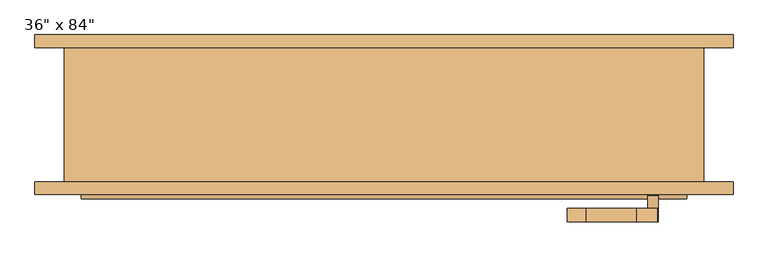
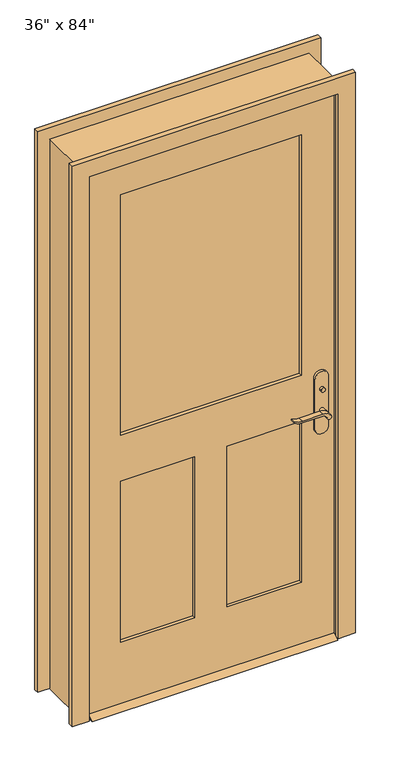
"""IFC4 building model written with IfcOpenShell, lengths in millimetres: door geometry."""

from ifc_helpers import new_model, si_unit, point, frame, frame_2d, origin, place, context, project, spatial, polyline, circle_curve, trimmed, segment, composite_curve, outline, extrude, faceted_brep, source, transform, mapped, element, save


def door_e879f077(model_context):
    return source(origin(), model_context, "Body", "SolidModel", [
        extrude(outline(polyline([(-63.5, 12.7), (-38.1, 0.0), (-123.825, 0.0), (-98.425, 12.7), (-63.5, 12.7)])), frame((-457.2, 0.0, 0.0), z_axis=(1.0, 0.0, 0.0), x_axis=(0.0, 1.0, 0.0)), (0.0, 0.0, 1.0), 914.4),
        extrude(outline(polyline([(411.4, -43.5), (411.4, -53.5), (401.4, -53.5), (401.4, -43.5), (411.4, -43.5)])), frame((0.0, 0.0, 981.9), z_axis=(0.0, 0.0, 1.0), x_axis=(1.0, 0.0, 0.0)), (0.0, 0.0, 1.0), 30.0),
        extrude(outline(composite_curve([segment(trimmed(circle_curve(frame_2d((996.9, 406.4)), 8.0), [point((996.9, 398.4))], [point((996.9, 414.4))], False, "CARTESIAN"), True, "CONTINUOUS"), segment(trimmed(circle_curve(frame_2d((996.9, 406.4)), 8.0), [point((996.9, 414.4))], [point((996.9, 398.4))], False, "CARTESIAN"), True, "CONTINUOUS")], self_intersect=False)), frame((0.0, -118.425, 0.0), z_axis=(0.0, 1.0, 0.0), x_axis=(0.0, 0.0, 1.0)), (0.0, 0.0, 1.0), 10.0),
        extrude(outline(composite_curve([segment(trimmed(circle_curve(frame_2d((897.1555521, 382.7324871)), 37.2832219), [point((919.0523287, 412.9081363))], [point((934.4, 381.0325667))], False, "CARTESIAN"), True, "CONTINUOUS"), segment(polyline([(934.4, 381.0325667), (934.4, 304.7564091)]), True, "CONTINUOUS"), segment(trimmed(circle_curve(frame_2d((1017.6850638, 304.8227909)), 83.2850902), [point((934.4, 304.7564091))], [point((939.4, 276.4))], True, "CARTESIAN"), True, "CONTINUOUS"), segment(polyline([(939.4, 276.4), (936.6135558, 276.4)]), True, "CONTINUOUS"), segment(trimmed(circle_curve(frame_2d((986.6709207, 308.3396612)), 59.3791355), [point((936.6135558, 276.4))], [point((927.4, 304.7564091))], False, "CARTESIAN"), True, "CONTINUOUS"), segment(polyline([(927.4, 304.7564091), (927.4, 381.0138099)]), True, "CONTINUOUS"), segment(trimmed(circle_curve(frame_2d((909.2738613, 381.0138099)), 18.1261387), [point((927.4, 381.0138099))], [point((914.4, 398.4))], True, "CARTESIAN"), True, "CONTINUOUS"), segment(trimmed(circle_curve(frame_2d((914.4, 406.4)), 8.0), [point((914.4, 398.4))], [point((919.0523287, 412.9081363))], False, "CARTESIAN"), True, "CONTINUOUS")], self_intersect=False)), frame((0.0, -23.5, 0.0), z_axis=(0.0, 1.0, 0.0), x_axis=(0.0, 0.0, 1.0)), (0.0, 0.0, 1.0), 20.0),
        extrude(outline(composite_curve([segment(trimmed(circle_curve(frame_2d((914.4, 406.4)), 8.0), [point((914.3999903, 398.4))], [point((919.0523287, 412.9081363))], False, "CARTESIAN"), True, "CONTINUOUS"), segment(trimmed(circle_curve(frame_2d((897.1555521, 382.7324871)), 37.2832219), [point((919.0523287, 412.9081363))], [point((934.4, 381.0325667))], False, "CARTESIAN"), True, "CONTINUOUS"), segment(polyline([(934.4, 381.0325667), (934.4, 304.7564091)]), True, "CONTINUOUS"), segment(trimmed(circle_curve(frame_2d((1017.6850638, 304.8227909)), 83.2850902), [point((934.4, 304.7564091))], [point((939.4, 276.4))], True, "CARTESIAN"), True, "CONTINUOUS"), segment(polyline([(939.4, 276.4), (936.6135558, 276.4)]), True, "CONTINUOUS"), segment(trimmed(circle_curve(frame_2d((986.6709207, 308.3396612)), 59.3791355), [point((936.6135558, 276.4))], [point((927.4, 304.7564091))], False, "CARTESIAN"), True, "CONTINUOUS"), segment(polyline([(927.4, 304.7564091), (927.4, 381.0138122)]), True, "CONTINUOUS"), segment(trimmed(circle_curve(frame_2d((909.2738682, 381.0138122)), 18.1261318), [point((927.4, 381.0138122))], [point((914.3999903, 398.4))], True, "CARTESIAN"), True, "CONTINUOUS")], self_intersect=False)), frame((0.0, -158.425, 0.0), z_axis=(0.0, 1.0, 0.0), x_axis=(0.0, 0.0, 1.0)), (0.0, 0.0, 1.0), 20.0),
        extrude(outline(composite_curve([segment(trimmed(circle_curve(frame_2d((914.4, 406.4)), 8.0), [point((914.4, 398.4))], [point((914.4, 414.4))], False, "CARTESIAN"), True, "CONTINUOUS"), segment(trimmed(circle_curve(frame_2d((914.4, 406.4)), 8.0), [point((914.4, 414.4))], [point((914.4, 398.4))], False, "CARTESIAN"), True, "CONTINUOUS")], self_intersect=False)), frame((0.0, -53.5, 0.0), z_axis=(0.0, 1.0, 0.0), x_axis=(0.0, 0.0, 1.0)), (0.0, 0.0, 1.0), 30.0),
        extrude(outline(composite_curve([segment(trimmed(circle_curve(frame_2d((914.4, 406.4)), 8.0), [point((914.4, 398.4))], [point((914.4, 414.4))], False, "CARTESIAN"), True, "CONTINUOUS"), segment(trimmed(circle_curve(frame_2d((914.4, 406.4)), 8.0), [point((914.4, 414.4))], [point((914.4, 398.4))], False, "CARTESIAN"), True, "CONTINUOUS")], self_intersect=False)), frame((0.0, -138.425, 0.0), z_axis=(0.0, 1.0, 0.0), x_axis=(0.0, 0.0, 1.0)), (0.0, 0.0, 1.0), 30.0),
        extrude(outline(composite_curve([segment(polyline([(844.4, 431.4), (1039.4, 431.4)]), True, "CONTINUOUS"), segment(trimmed(circle_curve(frame_2d((1039.4, 406.4)), 25.0), [point((1039.4, 431.4))], [point((1039.4, 381.4))], False, "CARTESIAN"), True, "CONTINUOUS"), segment(polyline([(1039.4, 381.4), (844.4, 381.4)]), True, "CONTINUOUS"), segment(trimmed(circle_curve(frame_2d((844.4, 406.4)), 25.0), [point((844.4, 381.4))], [point((844.4, 431.4))], False, "CARTESIAN"), True, "CONTINUOUS")], self_intersect=False)), frame((0.0, -63.5, 0.0), z_axis=(0.0, 1.0, 0.0), x_axis=(0.0, 0.0, 1.0)), (0.0, 0.0, 1.0), 10.0),
        extrude(outline(composite_curve([segment(polyline([(844.4, 431.4), (1039.4, 431.4)]), True, "CONTINUOUS"), segment(trimmed(circle_curve(frame_2d((1039.4, 406.4)), 25.0), [point((1039.4, 431.4))], [point((1039.4, 381.4))], False, "CARTESIAN"), True, "CONTINUOUS"), segment(polyline([(1039.4, 381.4), (844.4, 381.4)]), True, "CONTINUOUS"), segment(trimmed(circle_curve(frame_2d((844.4, 406.4)), 25.0), [point((844.4, 381.4))], [point((844.4, 431.4))], False, "CARTESIAN"), True, "CONTINUOUS")], self_intersect=False)), frame((0.0, -108.425, 0.0), z_axis=(0.0, 1.0, 0.0), x_axis=(0.0, 0.0, 1.0)), (0.0, 0.0, 1.0), 10.0),
        extrude(outline(polyline([(2133.6, -457.2), (12.7, -457.2), (12.7, 457.2), (2133.6, 457.2), (2133.6, -457.2)]), holes=[polyline([(1066.8, -336.55), (2012.95, -336.55), (2012.95, 336.55), (1066.8, 336.55), (1066.8, -336.55)]), polyline([(885.825, -60.325), (254.0, -60.325), (254.0, -336.55), (885.825, -336.55), (885.825, -60.325)]), polyline([(885.825, 336.55), (254.0, 336.55), (254.0, 60.325), (885.825, 60.325), (885.825, 336.55)])]), frame((0.0, -98.425, 0.0), z_axis=(0.0, 1.0, 0.0), x_axis=(0.0, 0.0, 1.0)), (0.0, 0.0, 1.0), 34.925),
        faceted_brep([(482.6, -98.425, 0.0), (457.2, -98.425, 0.0), (457.2, -63.5, 0.0), (444.5, -63.5, 0.0), (444.5, -28.575, 0.0), (457.2, -28.575, 0.0), (457.2, 104.775, 0.0), (482.6, 104.775, 0.0), (482.6, 104.775, 2159.0), (482.6, -98.425, 2159.0), (457.2, 104.775, 2133.6), (-457.2, 104.775, 2133.6), (-457.2, 104.775, 0.0), (-482.6, 104.775, 0.0), (-482.6, 104.775, 2159.0), (457.2, -28.575, 2133.6), (444.5, -28.575, 2120.9), (-444.5, -28.575, 2120.9), (-444.5, -28.575, 0.0), (-457.2, -28.575, 0.0), (-457.2, -28.575, 2133.6), (444.5, -63.5, 2120.9), (457.2, -63.5, 2133.6), (-457.2, -63.5, 2133.6), (-457.2, -63.5, 0.0), (-444.5, -63.5, 0.0), (-444.5, -63.5, 2120.9), (457.2, -98.425, 2133.6), (-482.6, -98.425, 2159.0), (-482.6, -98.425, 0.0), (-457.2, -98.425, 0.0), (-457.2, -98.425, 2133.6)], [[[0, 1, 2, 3, 4, 5, 6, 7]], [[7, 8, 9, 0]], [[6, 10, 11, 12, 13, 14, 8, 7]], [[5, 15, 10, 6]], [[4, 16, 17, 18, 19, 20, 15, 5]], [[3, 21, 16, 4]], [[2, 22, 23, 24, 25, 26, 21, 3]], [[1, 27, 22, 2]], [[0, 9, 28, 29, 30, 31, 27, 1]], [[8, 14, 28, 9]], [[15, 20, 11, 10]], [[21, 26, 17, 16]], [[27, 31, 23, 22]], [[29, 13, 12, 19, 18, 25, 24, 30]], [[14, 13, 29, 28]], [[20, 19, 12, 11]], [[26, 25, 18, 17]], [[31, 30, 24, 23]]]),
        extrude(outline(polyline([(-60.325, -75.1416667), (-60.325, -86.7833333), (-336.55, -86.7833333), (-336.55, -75.1416667), (-60.325, -75.1416667)])), frame((0.0, 0.0, 254.0), z_axis=(0.0, 0.0, 1.0), x_axis=(1.0, 0.0, 0.0)), (0.0, 0.0, 1.0), 631.825),
        extrude(outline(polyline([(336.55, -75.1416667), (336.55, -86.7833333), (60.325, -86.7833333), (60.325, -75.1416667), (336.55, -75.1416667)])), frame((0.0, 0.0, 254.0), z_axis=(0.0, 0.0, 1.0), x_axis=(1.0, 0.0, 0.0)), (0.0, 0.0, 1.0), 631.825),
        extrude(outline(polyline([(336.55, -77.47), (336.55, -84.455), (-336.55, -84.455), (-336.55, -77.47), (336.55, -77.47)])), frame((0.0, 0.0, 1066.8), z_axis=(0.0, 0.0, 1.0), x_axis=(1.0, 0.0, 0.0)), (0.0, 0.0, 1.0), 946.15),
        extrude(outline(polyline([(0.0, -463.55), (2139.95, -463.55), (2139.95, 463.55), (0.0, 463.55), (0.0, 527.05), (2203.45, 527.05), (2203.45, -527.05), (0.0, -527.05), (0.0, -463.55)])), frame((0.0, 104.775, 0.0), z_axis=(0.0, 1.0, 0.0), x_axis=(0.0, 0.0, 1.0)), (0.0, 0.0, 1.0), 19.05),
        extrude(outline(polyline([(0.0, -463.55), (2139.95, -463.55), (2139.95, 463.55), (0.0, 463.55), (0.0, 527.05), (2203.45, 527.05), (2203.45, -527.05), (0.0, -527.05), (0.0, -463.55)])), frame((0.0, -117.475, 0.0), z_axis=(0.0, 1.0, 0.0), x_axis=(0.0, 0.0, 1.0)), (0.0, 0.0, 1.0), 19.05),
    ])


if __name__ == "__main__":
    model = new_model("IFC4")
    model_context = context("Model", 3, world=origin())
    ifc_project = project(units=[si_unit("LENGTHUNIT", "METRE", prefix="MILLI")], contexts=[model_context])
    site = spatial("IfcSite", under=ifc_project)
    building = spatial("IfcBuilding", under=site)
    placement = place(None, origin())
    door_shape = door_e879f077(model_context)
    element("IfcDoor", 1, ObjectType="36\" x 84\"", at=placement, inside=building, context=model_context, shape_type="MappedRepresentation", body=[
        mapped(door_shape, transform((0.0, 0.0, 0.0), x_axis=(1.0, 0.0, 0.0), y_axis=(0.0, 1.0, 0.0), z_axis=(0.0, 0.0, 1.0))),
    ])
    save(model, "model.ifc")

# Revit data of these elements
# Type "36\" x 84\""
#   Type Mark = "15"
#   Assembly Code = "B2030100"
#   Analytic Construction = "French door, wood frame with single glass"
#   Top Rail = 0' - 4 3/4"
#   Threshold Offset [instance default] = 0' - 0 1/2"
#   Thickness = 0' - 1 3/8"
#   Thermal Resistance (R) = 1.0696 (h·ft²·°F)/BTU
#   Swing Angle [instance default] = 90.00°
#   Stiles = 0' - 4 3/4"
#   Rough Width = 3' - 2"
#   Rough Height = 7' - 1"
#   Lock Rail = 0' - 7 1/8"
#   Height = 7' - 0"
#   Width = 3' - 0"
#   Heat Transfer Coefficient (U) = 0.9350 BTU/(h·ft²·°F)
#   Door Offset [instance default] = 0' - 0"
#   Bottom Rail = 0' - 9 1/2"
#   Threshold [instance default] = yes
#   Function = 1
#   Exterior Trim [instance default] = yes
#   Trim Material = Cherry
#   Threshold Material = Cherry
#   Panel Material = Cherry
#   Glazing = Glass
#   Frame Material = Cherry
#   Door Handle Material = Aluminum
#   Visual Light Transmittance = 0
#   Solar Heat Gain Coefficient = 0
#   Wall Closure = (empty or 0)
#   Construction Type = (empty or 0)
# Element 1 (IfcDoor, "36\" x 84\"")
#   Materials on its faces: "Cherry", "Aluminum", "Glass"
# Materials
#   "Cherry": class "Wood", colour RGB 226 177 128, transparency 0, Description = "Prunus Serotina", Cost = 0
#   "Glass": class "Glass", colour RGB 0 128 192, transparency 0.75, Description = "Soda Lime Glass", Cost = 0
#   "Aluminum": class "Metal", colour RGB 247 247 247, transparency 0, Description = "Aluminum 6061", Cost = 0
